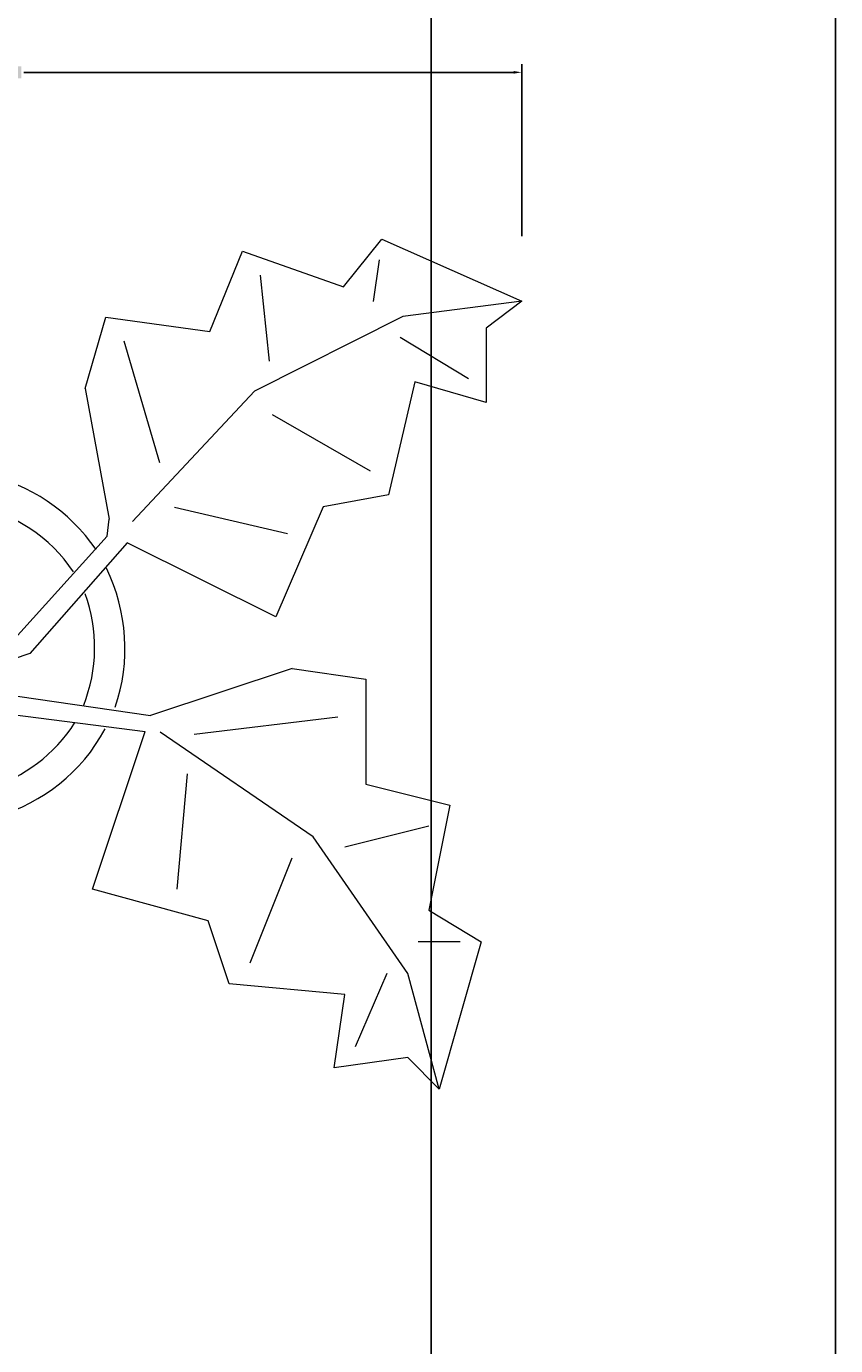
# Model space of a CAD drawing. Units: inches. Extents: x -301 to 715, y -607 to 364.
# Tile 89 of 141: x 115 to 133, y -260 to -231. Entities that reach past the tile are written whole.
import ezdxf

# ---------------------------------------------------------------- set-up
doc = ezdxf.new("R2010")
doc.units = ezdxf.units.IN
doc.header["$MEASUREMENT"] = 0
doc.layers.add('A-ANNO-DIMS', color=2, linetype='Continuous', lineweight=18)
doc.layers.add('L-PLNT', color=94, linetype='Continuous', lineweight=13)
doc.styles.get("Standard").update_dxf_attribs({"font": 'arial.ttf'})
doc.dimstyles.get("Standard").update_dxf_attribs({"dimtxt": 0.18, "dimasz": 0.18, "dimexe": 0.18, "dimexo": 0.0625, "dimgap": 0.09, "dimtad": 0, "dimtih": 1, "dimtoh": 1, "dimdec": 1, "dimzin": 0, "dimdsep": 46, "dimlunit": 4, "dimtxsty": 'Standard', "dimcen": 0.09, "dimclrd": 3, "dimclre": 4, "dimclrt": 6, "dimadec": 0, "dimazin": 0, "dimtfac": 1, "dimtdec": 1, "dimtofl": 0, "dimtmove": 0, "dimatfit": 3, "dimfxl": 1, "dimtfill": 2, "dimtfillclr": 51, "dimtolj": 1, "dimtzin": 0, "dimarcsym": 0})

# ---------------------------------------------------------------- blocks, each defined once
blk = doc.blocks.new('Plant - Rubber or Philodendron')
for p, q in [((13.3837, 12.301), (14.68, 13.9039)), ((14.68, 13.9039), (19.3848, 11.8146)), ((8.8871, 10.7908), (9.9809, 13.4933)), ((9.9809, 13.4933), (13.3837, 12.301)), ((14.5816, 13.2037), (14.3848, 11.8033)), ((10.5828, 12.6946), (10.8893, 9.7953)), ((-14.8639, 10.7964), (-12.6195, 11.8975)), ((-12.6195, 11.8975), (-12.1909, 9.4345)), ((19.3848, 11.8146), (15.3859, 11.3055)), ((19.3848, 11.8146), (18.1868, 10.9119)), ((-16.2005, 11.4774), (-13.9899, 8.1064)), ((-16.2005, 11.4774), (-14.8639, 10.7964)), ((-16.0159, 6.3329), (-16.2005, 11.4774)), ((4.6914, 8.8812), (5.3859, 11.2828)), ((5.3859, 11.2828), (8.8871, 10.7908)), ((15.3859, 11.3055), (10.3916, 8.7942)), ((-13.3174, 8.325), (-13.0735, 11.0065)), ((18.1868, 10.9119), (18.1925, 8.4119)), ((-12.1909, 9.4345), (-8.3829, 10.3)), ((-8.3829, 10.3), (-7.0549, 8.501)), ((5.9878, 10.4842), (7.1971, 6.3869)), ((15.2875, 10.6053), (17.5907, 9.2105)), ((-8.8369, 9.409), (-9.0894, 5.6095)), ((4.6914, 8.8812), (5.5014, 4.4831)), ((15.7909, 9.1065), (14.8995, 5.3044)), ((18.1925, 8.4119), (15.7909, 9.1065)), ((-7.0549, 8.501), (-3.0284, 8.6941)), ((-3.0284, 8.6941), (-3.0709, 3.1041)), ((10.3916, 8.7942), (6.2847, 4.4028)), ((-13.9899, 8.1064), (-9.5434, 4.7185)), ((14.2977, 6.1031), (10.9934, 7.9956)), ((-4.8529, 4.012), (-5.7184, 7.82)), ((-15.3434, 6.5514), (-13.9984, 6.9884)), ((-14.0069, 5.8704), (-16.0159, 6.3329)), ((-13.5868, 2.2894), (-14.0069, 5.8704)), ((7.7005, 4.8881), (11.5025, 3.9967)), ((12.7005, 4.8994), (11.1089, 1.1958)), ((14.8995, 5.3044), (12.7005, 4.8994)), ((-13.1329, 3.1804), (-10.6614, 4.727)), ((-9.5434, 4.7185), (-4.1917, 2.9888)), ((5.4346, 3.9146), (5.5014, 4.4831)), ((2.1141, 0.2298), (5.4346, 3.9146)), ((6.1032, 3.6844), (2.8262, -0.031)), ((11.1089, 1.1958), (6.1032, 3.6844)), ((-9.1318, 0.0195), (-5.9793, 2.9025)), ((-3.0709, 3.1041), (0.0797, 2.3163)), ((-10.6784, 2.491), (-13.5868, 2.2894)), ((-9.5858, -0.8715), (-10.6784, 2.491)), ((-3.5248, 2.2131), (-3.3011, 2.4355)), ((-3.3011, 2.4355), (-0.5306, 1.7947)), ((0.0797, 2.3163), (0.4866, -0.031)), ((-7.1228, -0.443), (-3.5248, 2.2131)), ((-0.5306, 1.7947), (-0.2255, -0.5527)), ((-0.5306, 1.7947), (-0.5306, 1.7947)), ((0.4866, -0.031), (2.1141, 0.2298)), ((-7.1228, -0.443), (-9.5858, -0.8715)), ((2.8262, -0.031), (1.3003, -0.5527)), ((-2.019, -3.6148), (-0.2255, -0.5527)), ((-0.9375, -3.1608), (0.5883, -0.8135)), ((0.5883, -0.8135), (2.2447, -2.0916)), ((1.3003, -0.5527), (2.4193, -1.4655)), ((11.6605, -0.5413), (6.895, -2.1175)), ((11.6605, -0.5413), (14.1354, -0.8948)), ((14.1354, -0.8948), (14.1354, -4.4304)), ((2.4193, -1.4655), (6.895, -2.1175)), ((2.2447, -2.0916), (6.7108, -2.6626)), ((8.3544, -2.7453), (13.1973, -2.1704)), ((4.943, -7.9659), (6.7108, -2.6626)), ((12.3677, -6.1981), (7.219, -2.6772)), ((-4.0579, -6.2781), (-0.9375, -3.1608)), ((-11.3237, -7.2629), (-9.7321, -3.5593)), ((-9.7321, -3.5593), (-4.7264, -6.0479)), ((-2.019, -3.6148), (-4.7264, -6.0479)), ((8.125, -4.0768), (7.7715, -7.9659)), ((14.1354, -4.4304), (16.9638, -5.1375)), ((16.9638, -5.1375), (16.2567, -8.673)), ((15.5496, -10.7943), (12.3677, -6.1981)), ((16.2567, -5.8446), (13.4283, -6.5517)), ((-6.3237, -7.2516), (-10.1257, -6.3602)), ((-4.1246, -6.8466), (-4.0579, -6.2781)), ((-9.0148, -11.1577), (-4.9047, -6.8122)), ((-3.3146, -11.2447), (-4.1246, -6.8466)), ((10.2463, -10.4408), (11.6605, -6.9053)), ((-13.5228, -7.6679), (-11.3237, -7.2629)), ((-14.4141, -11.4699), (-13.5228, -7.6679)), ((8.8321, -9.0266), (4.943, -7.9659)), ((-12.921, -8.4665), (-9.6166, -10.359)), ((-4.611, -12.8477), (-5.8203, -8.7504)), ((16.2567, -8.673), (18.0245, -9.7337)), ((9.5392, -11.1479), (8.8321, -9.0266)), ((17.3174, -9.7337), (15.9032, -9.7337)), ((18.0245, -9.7337), (16.6103, -14.6834)), ((-16.8157, -10.7754), (-14.4141, -11.4699)), ((-16.8101, -13.2754), (-16.8157, -10.7754)), ((14.8425, -10.7943), (13.7819, -13.2692)), ((16.6103, -14.6834), (15.5496, -10.7943)), ((-14.0091, -13.669), (-9.0148, -11.1577)), ((-3.3146, -11.2447), (-4.0092, -13.6463)), ((13.4283, -11.5015), (9.5392, -11.1479)), ((13.0748, -13.9763), (13.4283, -11.5015)), ((-13.9107, -12.9688), (-16.2139, -11.574)), ((-9.206, -15.0581), (-9.5126, -12.1588)), ((-18.008, -14.1781), (-16.8101, -13.2754)), ((-7.5103, -13.1543), (-8.6042, -15.8568)), ((-4.0092, -13.6463), (-7.5103, -13.1543)), ((-18.008, -14.1781), (-14.0091, -13.669)), ((15.5496, -13.6228), (13.0748, -13.9763)), ((16.6103, -14.6834), (15.5496, -13.6228)), ((-13.3032, -16.2674), (-18.008, -14.1781)), ((-13.2048, -15.5672), (-13.008, -14.1668)), ((-12.0069, -14.6645), (-13.3032, -16.2674)), ((-8.6042, -15.8568), (-12.0069, -14.6645))]:
    blk.add_line(p, q)
for centre, radius, start, end in [((0, 0), 6.1275, 34.37569, 120.1028), ((-0.0601, -0.2075), 5.2461, 33.82192, 124.9414), ((-0.098, 0.1364), 6.1288, 341.2017, 26.09184), ((-0.2664, 0.1682), 5.2775, 338.4094, 20.03007), ((0.0308, 0.1664), 5, 168.1647, 238.6725), ((0.0308, 0.1664), 6, 178.6147, 235.1169), ((-0.0234, 0.3825), 6.1492, 242.5812, 331.2714), ((-0.1102, 0.4886), 5.2883, 247.3711, 327.472)]:
    blk.add_arc(centre, radius, start, end)
blk = doc.blocks.new('*D106')
at = {"layer": 'A-ANNO-DIMS', "color": 4, "lineweight": -2, "transparency": 16777216}
for p, q in [((101.18, -235.449), (101.18, -231.622)), ((125.91, -235.449), (125.91, -231.622))]:
    blk.add_line(p, q, dxfattribs=at)
at = {"layer": 'A-ANNO-DIMS', "color": 3, "lineweight": -2, "transparency": 16777216}
for p, q in [((101.36, -231.802), (112.261, -231.802)), ((125.73, -231.802), (114.829, -231.802))]:
    blk.add_line(p, q, dxfattribs=at)
at = {"layer": 'A-ANNO-DIMS', "color": 3, "transparency": 16777216}
for points in [[(101.36, -231.772), (101.36, -231.832), (101.18, -231.802)], [(125.73, -231.772), (125.73, -231.832), (125.91, -231.802)]]:
    blk.add_solid(points, dxfattribs=at)
at = {"layer": 'Defpoints', "color": 0, "transparency": 16777216}
for p in [(125.91, -231.802), (101.18, -235.511), (125.91, -235.511)]:
    blk.add_point(p, dxfattribs=at)
at = {"layer": 'A-ANNO-DIMS', "color": 6, "transparency": 16777216, "insert": (113.545, -231.802), "char_height": 0.18, "attachment_point": 5, "bg_fill": 1, "box_fill_scale": 1.25, "bg_fill_color": 51, "bg_fill_transparency": 0}
blk.add_mtext('\\A1;PLANT 2\'-0 1/2" TYP.', dxfattribs=at)
blk = doc.blocks.new('*D156')
at = {"layer": 'A-ANNO-DIMS', "color": 4, "lineweight": -2, "transparency": 16777216}
for p, q in [((123.897, -214.88), (123.897, -296.865)), ((132.897, -223.88), (132.897, -296.865))]:
    blk.add_line(p, q, dxfattribs=at)
at = {"layer": 'A-ANNO-DIMS', "color": 3, "lineweight": -2, "transparency": 16777216}
for p, q in [((124.077, -296.685), (128.067, -296.685)), ((132.717, -296.685), (128.726, -296.685))]:
    blk.add_line(p, q, dxfattribs=at)
at = {"layer": 'A-ANNO-DIMS', "color": 3, "transparency": 16777216}
for points in [[(124.077, -296.655), (124.077, -296.715), (123.897, -296.685)], [(132.717, -296.655), (132.717, -296.715), (132.897, -296.685)]]:
    blk.add_solid(points, dxfattribs=at)
at = {"layer": 'Defpoints', "color": 0, "transparency": 16777216}
for p in [(123.897, -214.818), (132.897, -223.818), (132.897, -296.685)]:
    blk.add_point(p, dxfattribs=at)
at = {"layer": 'A-ANNO-DIMS', "color": 6, "transparency": 16777216, "insert": (128.397, -296.685), "char_height": 0.18, "attachment_point": 5, "bg_fill": 1, "box_fill_scale": 1.25, "bg_fill_color": 51, "bg_fill_transparency": 0}
blk.add_mtext('\\A1;0\'-9"', dxfattribs=at)

msp = doc.modelspace()

# ---------------------------------------------------------------- block references
at = {"layer": 'L-PLNT', "xscale": 0.6613521884636907, "yscale": 0.6613521884636907, "zscale": 0.6613521884636907}
msp.add_blockref('Plant - Rubber or Philodendron', (113.09, -244.707), dxfattribs=at)

# ---------------------------------------------------------------- dimensions: what is measured, and where the dimension line sits
at = {"layer": 'A-ANNO-DIMS'}
dim = msp.add_linear_dim(base=(132.897, -296.685), p1=(123.897, -214.818), p2=(132.897, -223.818), dimstyle='Standard', override={"dimdec": 1, "dimlfac": 1, "dimrnd": 0, "dimzin": 1, "dimdsep": 46, "dimlunit": 4, "dimfrac": 2}, dxfattribs=at)
dim.commit()
dim.dimension.update_dxf_attribs({"geometry": '*D156', "text_midpoint": (128.397, -296.685)})
dim = msp.add_linear_dim(base=(125.91, -231.802), p1=(101.18, -235.511), p2=(125.91, -235.511), text='PLANT <> TYP.', dimstyle='Standard', override={"dimdec": 1, "dimlfac": 1, "dimrnd": 0, "dimzin": 1, "dimdsep": 46, "dimlunit": 4, "dimfrac": 2}, dxfattribs=at)
dim.commit()
dim.dimension.update_dxf_attribs({"geometry": '*D106', "text_midpoint": (113.545, -231.802)})

doc.saveas('drawing.dxf')
